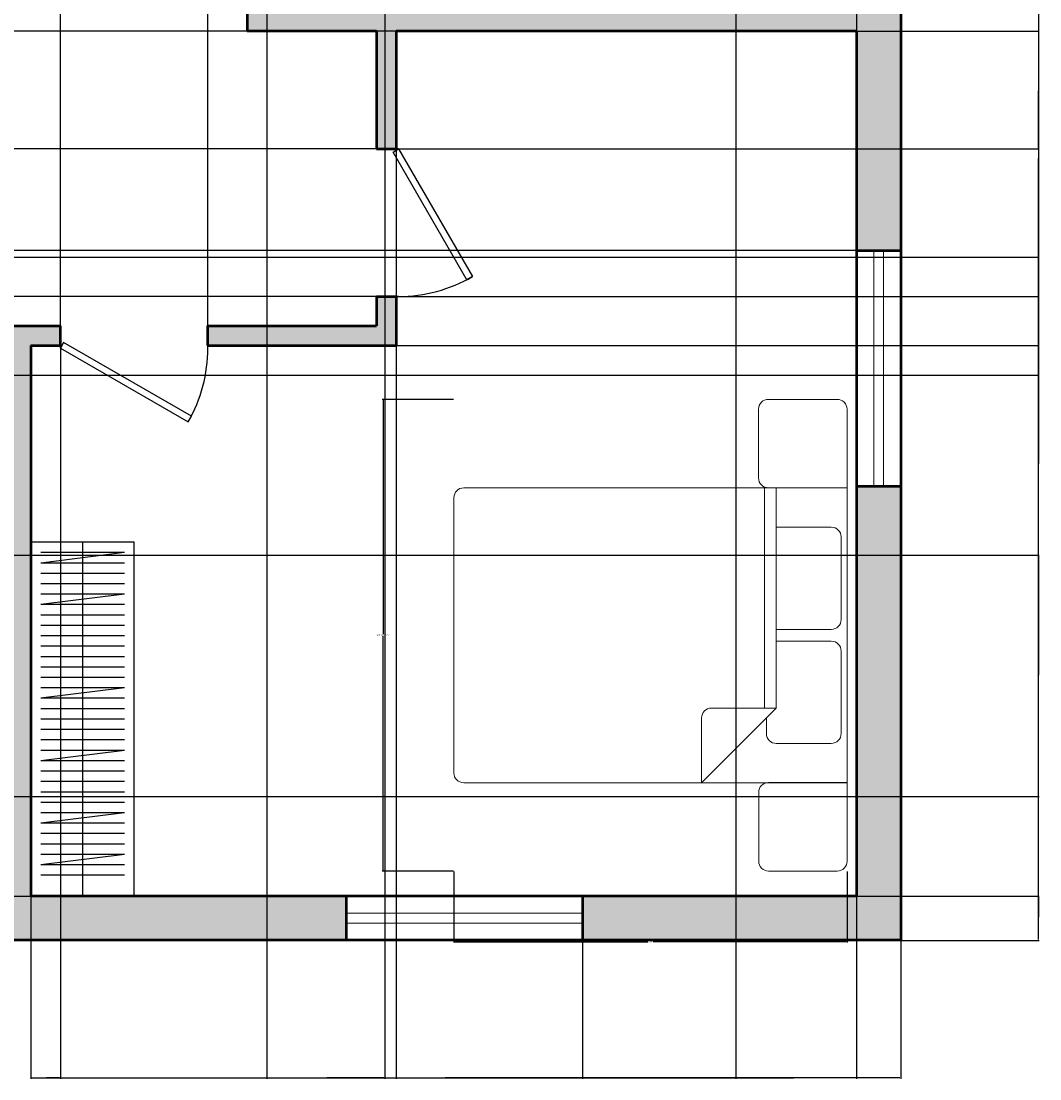
# Model space of a CAD drawing. Units: inches. Extents: x 1869 to 2483, y 2084 to 2479.
# Tile 6 of 7: x 2276 to 2483, y 2084 to 2299. Entities that reach past the tile are written whole.
import ezdxf

# ---------------------------------------------------------------- set-up
doc = ezdxf.new("R2010")
doc.units = ezdxf.units.IN
for name, color, linetype, lineweight in [('A-ANNO-DIMS', 2, 'Continuous', 18), ('A-DOOR', 3, 'Continuous', 25), ('A-FLOR-CASE', 9, 'Continuous', 25), ('A-FURN', 8, 'Continuous', 18), ('A-GLAZ', 4, 'Continuous', 18), ('A-WALL', 7, 'Continuous', 50)]:
    doc.layers.add(name, color=color, linetype=linetype, lineweight=lineweight)
doc.layers.add('A-WALL-PATT', color=18, linetype='Continuous', lineweight=13, true_color=0x000000)
doc.styles.get("Standard").update_dxf_attribs({"font": 'arial.ttf'})
doc.dimstyles.get("Standard").update_dxf_attribs({"dimtxt": 0.18, "dimasz": 0.18, "dimexe": 0.18, "dimexo": 0.0625, "dimgap": 0.09, "dimtad": 0, "dimtih": 1, "dimtoh": 1, "dimdec": 4, "dimzin": 0, "dimdsep": 46, "dimtxsty": 'Standard', "dimcen": 0.09, "dimadec": 0, "dimazin": 0, "dimtfac": 1, "dimtdec": 4, "dimtofl": 0, "dimtmove": 0, "dimatfit": 3, "dimfxl": 1, "dimtolj": 1, "dimtzin": 0, "dimarcsym": 0})

# ---------------------------------------------------------------- blocks, each defined once
blk = doc.blocks.new('Bed - Queen')
for p, q in [((0, -78), (0, 0)), ((0, 0), (60, 0)), ((60, 0), (60, -78)), ((10, -1.2), (26.8, -1.2)), ((33.2, -1.2), (50, -1.2)), ((8, -14.4), (8, -3.2)), ((28.8, -3.2), (28.8, -14.4)), ((31.2, -14.4), (31.2, -3.2)), ((52, -3.2), (52, -14.4)), ((0, -14.4), (44.8, -14.4)), ((60, -29.6), (44.8, -14.4)), ((44.8, -14.4), (44.8, -27.6)), ((44.8, -16.8), (0, -16.8)), ((50, -16.4), (46.8, -16.4)), ((46.8, -29.6), (60, -29.6)), ((58, -80), (2, -80))]:
    blk.add_line(p, q)
for points in [[(0, 0), (-16, 0, 0.414214), (-18, -2), (-18, -16, 0.414214), (-16, -18), (-2, -18, 0.414214), (0, -16)], [(75.96, 0.02), (59.96, 0.02), (59.96, -15.98, 0.414214), (61.96, -17.98), (75.96, -17.98, 0.414214), (77.96, -15.98), (77.96, -1.98, 0.414214)]]:
    blk.add_lwpolyline(points, format="xyb", close=True)
for centre, start, end in [((10, -3.2), 90, 180), ((26.8, -3.2), 0, 90), ((33.2, -3.2), 90, 180), ((50, -3.2), 0, 90), ((50, -14.4), 270, 0), ((46.8, -27.6), 180, 270), ((2, -78), 180, 270), ((58, -78), 270, 0)]:
    blk.add_arc(centre, 2, start, end)
blk = doc.blocks.new('*U13')
for p, q in [((0, 0), (0, 6)), ((40, 0), (40, 6))]:
    blk.add_line(p, q)
blk.add_lwpolyline([(0, 0), (34.64, -20), (35.52, -18.48), (0.87, 1.52)], close=True)
blk.add_arc((0, 0), 40, 330, 0)
blk = doc.blocks.new('*U10')
for p, q in [((0, 0), (0, -6)), ((40, 0), (40, -6))]:
    blk.add_line(p, q)
blk.add_lwpolyline([(0, 0), (34.64, 20), (35.52, 18.48), (0.87, -1.52)], close=True)
blk.add_arc((0, 0), 40, 0, 30)
blk = doc.blocks.new('WIN-GLAZING-48IN')
for p, q in [((0, 2), (48, 2)), ((0, 0), (48, 0))]:
    blk.add_line(p, q)
blk = doc.blocks.new('*D19')
at = {"layer": 'A-ANNO-DIMS', "color": 0, "lineweight": -2, "transparency": 16777216}
for p, q in [((2364.09, 2221.78), (2349.57, 2221.78)), ((2349.75, 2221.6), (2349.75, 2173.99)), ((2349.75, 2126), (2349.75, 2173.62)), ((2364.09, 2125.82), (2349.57, 2125.82))]:
    blk.add_line(p, q, dxfattribs=at)
at = {"layer": 'A-ANNO-DIMS', "color": 0, "transparency": 16777216}
for points in [[(2349.72, 2221.6), (2349.78, 2221.6), (2349.75, 2221.78)], [(2349.72, 2126), (2349.78, 2126), (2349.75, 2125.82)]]:
    blk.add_solid(points, dxfattribs=at)
at = {"layer": 'Defpoints', "color": 0, "transparency": 16777216}
for p in [(2364.15, 2221.78), (2349.75, 2125.82), (2364.15, 2125.82)]:
    blk.add_point(p, dxfattribs=at)
at = {"layer": 'A-ANNO-DIMS', "color": 0, "transparency": 16777216, "insert": (2349.75, 2173.8), "char_height": 0.18, "attachment_point": 5}
blk.add_mtext('\\A1;QUEEN BED SET 96 TYP.', dxfattribs=at)
blk = doc.blocks.new('*D20')
at = {"layer": 'A-ANNO-DIMS', "color": 0, "lineweight": -2, "transparency": 16777216}
for p, q in [((2364.15, 2125.76), (2364.15, 2111.25)), ((2444.17, 2125.76), (2444.17, 2111.25)), ((2364.33, 2111.43), (2403.63, 2111.43)), ((2443.99, 2111.43), (2404.69, 2111.43))]:
    blk.add_line(p, q, dxfattribs=at)
at = {"layer": 'A-ANNO-DIMS', "color": 0, "transparency": 16777216}
for points in [[(2364.33, 2111.46), (2364.33, 2111.4), (2364.15, 2111.43)], [(2443.99, 2111.46), (2443.99, 2111.4), (2444.17, 2111.43)]]:
    blk.add_solid(points, dxfattribs=at)
at = {"layer": 'Defpoints', "color": 0, "transparency": 16777216}
for p in [(2364.15, 2125.82), (2444.17, 2125.82), (2444.17, 2111.43)]:
    blk.add_point(p, dxfattribs=at)
at = {"layer": 'A-ANNO-DIMS', "color": 0, "transparency": 16777216, "insert": (2404.16, 2111.43), "char_height": 0.18, "attachment_point": 5}
blk.add_mtext('\\A1;80 TYP.', dxfattribs=at)
blk = doc.blocks.new('*D42')
at = {"layer": 'A-ANNO-DIMS', "color": 0, "lineweight": -2, "transparency": 16777216}
for p, q in [((2278.08, 2120.66), (2278.08, 2083.54)), ((2446.08, 2120.66), (2446.08, 2083.54)), ((2278.26, 2083.72), (2361.8, 2083.72)), ((2445.9, 2083.72), (2362.36, 2083.72))]:
    blk.add_line(p, q, dxfattribs=at)
at = {"layer": 'A-ANNO-DIMS', "color": 0, "transparency": 16777216}
for points in [[(2278.26, 2083.75), (2278.26, 2083.69), (2278.08, 2083.72)], [(2445.9, 2083.75), (2445.9, 2083.69), (2446.08, 2083.72)]]:
    blk.add_solid(points, dxfattribs=at)
at = {"layer": 'Defpoints', "color": 0, "transparency": 16777216}
for p in [(2278.08, 2120.72), (2446.08, 2120.72), (2446.08, 2083.72)]:
    blk.add_point(p, dxfattribs=at)
at = {"layer": 'A-ANNO-DIMS', "color": 0, "transparency": 16777216, "insert": (2362.08, 2083.72), "char_height": 0.18, "attachment_point": 5}
blk.add_mtext('\\A1;168', dxfattribs=at)
blk = doc.blocks.new('*D48')
at = {"layer": 'A-ANNO-DIMS', "color": 0, "lineweight": -2, "transparency": 16777216}
for p, q in [((2446.14, 2296.72), (2483.26, 2296.72)), ((2483.08, 2296.54), (2483.08, 2208.91)), ((2483.08, 2120.9), (2483.08, 2208.54)), ((2446.14, 2120.72), (2483.26, 2120.72))]:
    blk.add_line(p, q, dxfattribs=at)
at = {"layer": 'A-ANNO-DIMS', "color": 0, "transparency": 16777216}
for points in [[(2483.05, 2296.54), (2483.11, 2296.54), (2483.08, 2296.72)], [(2483.05, 2120.9), (2483.11, 2120.9), (2483.08, 2120.72)]]:
    blk.add_solid(points, dxfattribs=at)
at = {"layer": 'Defpoints', "color": 0, "transparency": 16777216}
for p in [(2446.08, 2296.72), (2483.08, 2296.72), (2446.08, 2120.72)]:
    blk.add_point(p, dxfattribs=at)
at = {"layer": 'A-ANNO-DIMS', "color": 0, "transparency": 16777216, "insert": (2483.08, 2208.72), "char_height": 0.18, "attachment_point": 5}
blk.add_mtext('\\A1;176', dxfattribs=at)
blk = doc.blocks.new('*D52')
at = {"layer": 'A-ANNO-DIMS', "color": 0, "lineweight": -2, "transparency": 16777216}
for p, q in [((2421.52, 2420.66), (2421.52, 2083.54)), ((2446.08, 2420.66), (2446.08, 2083.54)), ((2421.7, 2083.72), (2433.34, 2083.72)), ((2445.9, 2083.72), (2434.27, 2083.72))]:
    blk.add_line(p, q, dxfattribs=at)
at = {"layer": 'A-ANNO-DIMS', "color": 0, "transparency": 16777216}
for points in [[(2421.7, 2083.75), (2421.7, 2083.69), (2421.52, 2083.72)], [(2445.9, 2083.75), (2445.9, 2083.69), (2446.08, 2083.72)]]:
    blk.add_solid(points, dxfattribs=at)
at = {"layer": 'Defpoints', "color": 0, "transparency": 16777216}
for p in [(2421.52, 2420.72), (2446.08, 2420.72), (2446.08, 2083.72)]:
    blk.add_point(p, dxfattribs=at)
at = {"layer": 'A-ANNO-DIMS', "color": 0, "transparency": 16777216, "insert": (2433.8, 2083.72), "char_height": 0.18, "attachment_point": 5}
blk.add_mtext('\\A1;24.555', dxfattribs=at)
blk = doc.blocks.new('*D56')
at = {"layer": 'A-ANNO-DIMS', "color": 0, "lineweight": -2, "transparency": 16777216}
for p, q in [((2390.29, 2111.66), (2390.29, 2083.54)), ((2455.08, 2111.66), (2455.08, 2083.54)), ((2390.47, 2083.72), (2422.29, 2083.72)), ((2454.9, 2083.72), (2423.08, 2083.72))]:
    blk.add_line(p, q, dxfattribs=at)
at = {"layer": 'A-ANNO-DIMS', "color": 0, "transparency": 16777216}
for points in [[(2390.47, 2083.75), (2390.47, 2083.69), (2390.29, 2083.72)], [(2454.9, 2083.75), (2454.9, 2083.69), (2455.08, 2083.72)]]:
    blk.add_solid(points, dxfattribs=at)
at = {"layer": 'Defpoints', "color": 0, "transparency": 16777216}
for p in [(2390.29, 2111.72), (2455.08, 2111.72), (2455.08, 2083.72)]:
    blk.add_point(p, dxfattribs=at)
at = {"layer": 'A-ANNO-DIMS', "color": 0, "transparency": 16777216, "insert": (2422.68, 2083.72), "char_height": 0.18, "attachment_point": 5}
blk.add_mtext('\\A1;64.79', dxfattribs=at)
blk = doc.blocks.new('*D57')
at = {"layer": 'A-ANNO-DIMS', "color": 0, "lineweight": -2, "transparency": 16777216}
for p, q in [((2446.02, 2296.72), (1868.9, 2296.72)), ((1869.08, 2296.54), (1869.08, 2274.58)), ((1869.08, 2252.25), (1869.08, 2274.22)), ((2446.02, 2252.07), (1868.9, 2252.07))]:
    blk.add_line(p, q, dxfattribs=at)
at = {"layer": 'A-ANNO-DIMS', "color": 0, "transparency": 16777216}
for points in [[(1869.05, 2296.54), (1869.11, 2296.54), (1869.08, 2296.72)], [(1869.05, 2252.25), (1869.11, 2252.25), (1869.08, 2252.07)]]:
    blk.add_solid(points, dxfattribs=at)
at = {"layer": 'Defpoints', "color": 0, "transparency": 16777216}
for p in [(1869.08, 2296.72), (2446.08, 2296.72), (2446.08, 2252.07)]:
    blk.add_point(p, dxfattribs=at)
at = {"layer": 'A-ANNO-DIMS', "color": 0, "transparency": 16777216, "insert": (1869.08, 2274.4), "char_height": 0.18, "attachment_point": 5}
blk.add_mtext('\\A1;44.65', dxfattribs=at)
blk = doc.blocks.new('*D60')
at = {"layer": 'A-ANNO-DIMS', "color": 0, "lineweight": -2, "transparency": 16777216}
for p, q in [((2352.46, 2242.72), (2483.26, 2242.72)), ((2483.08, 2242.54), (2483.08, 2237.91)), ((2483.08, 2232.9), (2483.08, 2237.54)), ((2352.46, 2232.72), (2483.26, 2232.72))]:
    blk.add_line(p, q, dxfattribs=at)
at = {"layer": 'A-ANNO-DIMS', "color": 0, "transparency": 16777216}
for points in [[(2483.05, 2242.54), (2483.11, 2242.54), (2483.08, 2242.72)], [(2483.05, 2232.9), (2483.11, 2232.9), (2483.08, 2232.72)]]:
    blk.add_solid(points, dxfattribs=at)
at = {"layer": 'Defpoints', "color": 0, "transparency": 16777216}
for p in [(2352.4, 2242.72), (2483.08, 2242.72), (2352.4, 2232.72)]:
    blk.add_point(p, dxfattribs=at)
at = {"layer": 'A-ANNO-DIMS', "color": 0, "transparency": 16777216, "insert": (2483.08, 2237.72), "char_height": 0.18, "attachment_point": 5}
blk.add_mtext('\\A1;10', dxfattribs=at)
blk = doc.blocks.new('*D61')
at = {"layer": 'A-ANNO-DIMS', "color": 0, "lineweight": -2, "transparency": 16777216}
for p, q in [((2352.4, 2296.66), (2352.4, 2083.54)), ((2446.08, 2296.66), (2446.08, 2083.54)), ((2352.58, 2083.72), (2398.85, 2083.72)), ((2445.9, 2083.72), (2399.63, 2083.72))]:
    blk.add_line(p, q, dxfattribs=at)
at = {"layer": 'A-ANNO-DIMS', "color": 0, "transparency": 16777216}
for points in [[(2352.58, 2083.75), (2352.58, 2083.69), (2352.4, 2083.72)], [(2445.9, 2083.75), (2445.9, 2083.69), (2446.08, 2083.72)]]:
    blk.add_solid(points, dxfattribs=at)
at = {"layer": 'Defpoints', "color": 0, "transparency": 16777216}
for p in [(2352.4, 2296.72), (2446.08, 2296.72), (2446.08, 2083.72)]:
    blk.add_point(p, dxfattribs=at)
at = {"layer": 'A-ANNO-DIMS', "color": 0, "transparency": 16777216, "insert": (2399.24, 2083.72), "char_height": 0.18, "attachment_point": 5}
blk.add_mtext('\\A1;93.68', dxfattribs=at)
blk = doc.blocks.new('*D63')
at = {"layer": 'A-ANNO-DIMS', "color": 0, "lineweight": -2, "transparency": 16777216}
for p, q in [((2348.34, 2272.72), (1868.9, 2272.72)), ((1869.08, 2272.54), (1869.08, 2257.91)), ((1869.08, 2242.9), (1869.08, 2257.54)), ((2348.34, 2242.72), (1868.9, 2242.72))]:
    blk.add_line(p, q, dxfattribs=at)
at = {"layer": 'A-ANNO-DIMS', "color": 0, "transparency": 16777216}
for points in [[(1869.05, 2272.54), (1869.11, 2272.54), (1869.08, 2272.72)], [(1869.05, 2242.9), (1869.11, 2242.9), (1869.08, 2242.72)]]:
    blk.add_solid(points, dxfattribs=at)
at = {"layer": 'Defpoints', "color": 0, "transparency": 16777216}
for p in [(1869.08, 2272.72), (2348.4, 2272.72), (2348.4, 2242.72)]:
    blk.add_point(p, dxfattribs=at)
at = {"layer": 'A-ANNO-DIMS', "color": 0, "transparency": 16777216, "insert": (1869.08, 2257.72), "char_height": 0.18, "attachment_point": 5}
blk.add_mtext('\\A1;30', dxfattribs=at)
blk = doc.blocks.new('*D64')
at = {"layer": 'A-ANNO-DIMS', "color": 0, "lineweight": -2, "transparency": 16777216}
for p, q in [((2284.08, 2236.79), (2284.08, 2479.07)), ((2284.26, 2478.89), (2298.86, 2478.89)), ((2313.9, 2478.89), (2299.3, 2478.89)), ((2314.08, 2236.79), (2314.08, 2479.07))]:
    blk.add_line(p, q, dxfattribs=at)
at = {"layer": 'A-ANNO-DIMS', "color": 0, "transparency": 16777216}
for points in [[(2284.26, 2478.92), (2284.26, 2478.86), (2284.08, 2478.89)], [(2313.9, 2478.92), (2313.9, 2478.86), (2314.08, 2478.89)]]:
    blk.add_solid(points, dxfattribs=at)
at = {"layer": 'Defpoints', "color": 0, "transparency": 16777216}
for p in [(2314.08, 2478.89), (2284.08, 2236.72), (2314.08, 2236.72)]:
    blk.add_point(p, dxfattribs=at)
at = {"layer": 'A-ANNO-DIMS', "color": 0, "transparency": 16777216, "insert": (2299.08, 2478.89), "char_height": 0.18, "attachment_point": 5}
blk.add_mtext('\\A1;30', dxfattribs=at)
blk = doc.blocks.new('*D68')
at = {"layer": 'A-ANNO-DIMS', "color": 0, "lineweight": -2, "transparency": 16777216}
for p, q in [((2010.14, 2250.72), (2483.26, 2250.72)), ((2483.08, 2250.54), (2483.08, 2238.9)), ((2483.08, 2226.9), (2483.08, 2238.54)), ((2010.14, 2226.72), (2483.26, 2226.72))]:
    blk.add_line(p, q, dxfattribs=at)
at = {"layer": 'A-ANNO-DIMS', "color": 0, "transparency": 16777216}
for points in [[(2483.05, 2250.54), (2483.11, 2250.54), (2483.08, 2250.72)], [(2483.05, 2226.9), (2483.11, 2226.9), (2483.08, 2226.72)]]:
    blk.add_solid(points, dxfattribs=at)
at = {"layer": 'Defpoints', "color": 0, "transparency": 16777216}
for p in [(2010.08, 2250.72), (2483.08, 2250.72), (2010.08, 2226.72)]:
    blk.add_point(p, dxfattribs=at)
at = {"layer": 'A-ANNO-DIMS', "color": 0, "transparency": 16777216, "insert": (2483.08, 2238.72), "char_height": 0.18, "attachment_point": 5}
blk.add_mtext('\\A1;24', dxfattribs=at)
blk = doc.blocks.new('*D73')
at = {"layer": 'A-ANNO-DIMS', "color": 0, "lineweight": -2, "transparency": 16777216}
for p, q in [((2200.14, 2120.72), (2483.26, 2120.72)), ((2483.08, 2120.54), (2483.08, 2116.41)), ((2483.08, 2111.9), (2483.08, 2116.04)), ((2200.14, 2111.72), (2483.26, 2111.72))]:
    blk.add_line(p, q, dxfattribs=at)
at = {"layer": 'A-ANNO-DIMS', "color": 0, "transparency": 16777216}
for points in [[(2483.05, 2120.54), (2483.11, 2120.54), (2483.08, 2120.72)], [(2483.05, 2111.9), (2483.11, 2111.9), (2483.08, 2111.72)]]:
    blk.add_solid(points, dxfattribs=at)
at = {"layer": 'Defpoints', "color": 0, "transparency": 16777216}
for p in [(2200.08, 2120.72), (2483.08, 2120.72), (2200.08, 2111.72)]:
    blk.add_point(p, dxfattribs=at)
at = {"layer": 'A-ANNO-DIMS', "color": 0, "transparency": 16777216, "insert": (2483.08, 2116.22), "char_height": 0.18, "attachment_point": 5}
blk.add_mtext('\\A1;9', dxfattribs=at)
blk = doc.blocks.new('*D76')
at = {"layer": 'A-ANNO-DIMS', "color": 0, "lineweight": -2, "transparency": 16777216}
for p, q in [((2455.14, 2429.72), (2483.26, 2429.72)), ((2483.08, 2429.54), (2483.08, 2270.91)), ((2483.08, 2111.9), (2483.08, 2270.54)), ((2455.14, 2111.72), (2483.26, 2111.72))]:
    blk.add_line(p, q, dxfattribs=at)
at = {"layer": 'A-ANNO-DIMS', "color": 0, "transparency": 16777216}
for points in [[(2483.05, 2429.54), (2483.11, 2429.54), (2483.08, 2429.72)], [(2483.05, 2111.9), (2483.11, 2111.9), (2483.08, 2111.72)]]:
    blk.add_solid(points, dxfattribs=at)
at = {"layer": 'Defpoints', "color": 0, "transparency": 16777216}
for p in [(2455.08, 2429.72), (2483.08, 2429.72), (2455.08, 2111.72)]:
    blk.add_point(p, dxfattribs=at)
at = {"layer": 'A-ANNO-DIMS', "color": 0, "transparency": 16777216, "insert": (2483.08, 2270.72), "char_height": 0.18, "attachment_point": 5}
blk.add_mtext('\\A1;318', dxfattribs=at)
blk = doc.blocks.new('*D77')
at = {"layer": 'A-ANNO-DIMS', "color": 0, "lineweight": -2, "transparency": 16777216}
for p, q in [((2326.08, 2336.66), (2326.08, 2083.54)), ((2350.08, 2336.66), (2350.08, 2083.54)), ((2326.26, 2083.72), (2337.86, 2083.72)), ((2349.9, 2083.72), (2338.3, 2083.72))]:
    blk.add_line(p, q, dxfattribs=at)
at = {"layer": 'A-ANNO-DIMS', "color": 0, "transparency": 16777216}
for points in [[(2326.26, 2083.75), (2326.26, 2083.69), (2326.08, 2083.72)], [(2349.9, 2083.75), (2349.9, 2083.69), (2350.08, 2083.72)]]:
    blk.add_solid(points, dxfattribs=at)
at = {"layer": 'Defpoints', "color": 0, "transparency": 16777216}
for p in [(2326.08, 2336.72), (2350.08, 2336.72), (2350.08, 2083.72)]:
    blk.add_point(p, dxfattribs=at)
at = {"layer": 'A-ANNO-DIMS', "color": 0, "transparency": 16777216, "insert": (2338.08, 2083.72), "char_height": 0.18, "attachment_point": 5}
blk.add_mtext('\\A1;24', dxfattribs=at)
blk = doc.blocks.new('*D80')
at = {"layer": 'A-ANNO-DIMS', "color": 0, "lineweight": -2, "transparency": 16777216}
for p, q in [((2278.08, 2232.66), (2278.08, 2083.54)), ((2284.08, 2232.66), (2284.08, 2083.54)), ((2278.26, 2083.72), (2280.93, 2083.72)), ((2283.9, 2083.72), (2281.23, 2083.72))]:
    blk.add_line(p, q, dxfattribs=at)
at = {"layer": 'A-ANNO-DIMS', "color": 0, "transparency": 16777216}
for points in [[(2278.26, 2083.75), (2278.26, 2083.69), (2278.08, 2083.72)], [(2283.9, 2083.75), (2283.9, 2083.69), (2284.08, 2083.72)]]:
    blk.add_solid(points, dxfattribs=at)
at = {"layer": 'Defpoints', "color": 0, "transparency": 16777216}
for p in [(2278.08, 2232.72), (2284.08, 2232.72), (2284.08, 2083.72)]:
    blk.add_point(p, dxfattribs=at)
at = {"layer": 'A-ANNO-DIMS', "color": 0, "transparency": 16777216, "insert": (2281.08, 2083.72), "char_height": 0.18, "attachment_point": 5}
blk.add_mtext('\\A1;6', dxfattribs=at)
blk = doc.blocks.new('*D81')
at = {"layer": 'A-ANNO-DIMS', "color": 0, "lineweight": -2, "transparency": 16777216}
for p, q in [((2352.46, 2296.72), (2483.26, 2296.72)), ((2483.08, 2296.54), (2483.08, 2284.9)), ((2483.08, 2272.9), (2483.08, 2284.54)), ((2352.46, 2272.72), (2483.26, 2272.72))]:
    blk.add_line(p, q, dxfattribs=at)
at = {"layer": 'A-ANNO-DIMS', "color": 0, "transparency": 16777216}
for points in [[(2483.05, 2296.54), (2483.11, 2296.54), (2483.08, 2296.72)], [(2483.05, 2272.9), (2483.11, 2272.9), (2483.08, 2272.72)]]:
    blk.add_solid(points, dxfattribs=at)
at = {"layer": 'Defpoints', "color": 0, "transparency": 16777216}
for p in [(2352.4, 2296.72), (2483.08, 2296.72), (2352.4, 2272.72)]:
    blk.add_point(p, dxfattribs=at)
at = {"layer": 'A-ANNO-DIMS', "color": 0, "transparency": 16777216, "insert": (2483.08, 2284.72), "char_height": 0.18, "attachment_point": 5}
blk.add_mtext('\\A1;24', dxfattribs=at)
blk = doc.blocks.new('*D93')
at = {"layer": 'A-ANNO-DIMS', "color": 0, "lineweight": -2, "transparency": 16777216}
for p, q in [((2103.9, 2190.06), (2483.26, 2190.06)), ((2483.08, 2189.88), (2483.08, 2165.72)), ((2483.08, 2141.19), (2483.08, 2165.36)), ((2103.9, 2141.01), (2483.26, 2141.01))]:
    blk.add_line(p, q, dxfattribs=at)
at = {"layer": 'A-ANNO-DIMS', "color": 0, "transparency": 16777216}
for points in [[(2483.05, 2189.88), (2483.11, 2189.88), (2483.08, 2190.06)], [(2483.05, 2141.19), (2483.11, 2141.19), (2483.08, 2141.01)]]:
    blk.add_solid(points, dxfattribs=at)
at = {"layer": 'Defpoints', "color": 0, "transparency": 16777216}
for p in [(2103.84, 2190.06), (2483.08, 2190.06), (2103.84, 2141.01)]:
    blk.add_point(p, dxfattribs=at)
at = {"layer": 'A-ANNO-DIMS', "color": 0, "transparency": 16777216, "insert": (2483.08, 2165.54), "char_height": 0.18, "attachment_point": 5}
blk.add_mtext('\\A1;49.05', dxfattribs=at)

msp = doc.modelspace()

# ---------------------------------------------------------------- hatches: boundary and pattern name
at = {"layer": 'A-WALL-PATT'}
h = msp.add_hatch(color=256, dxfattribs=at)
h.dxf.hatch_style = 1
h.paths.add_polyline_path([(2352.3982, 2296.7235), (2446.0799, 2296.7235), (2446.0799, 2252.0706), (2455.0799, 2252.0706), (2455.0799, 2429.7235), (2421.5248, 2429.7235), (2421.5248, 2420.7235), (2446.0799, 2420.7235), (2446.0799, 2300.7235), (2326.0799, 2300.7235), (2326.0799, 2306.7235), (2322.0799, 2306.7235), (2322.0799, 2296.7235), (2348.3982, 2296.7235), (2348.3982, 2272.7235), (2352.3982, 2272.7235)])
h = msp.add_hatch(color=256, dxfattribs=at)
h.dxf.hatch_style = 1
h.paths.add_polyline_path([(2352.3982, 2242.7235), (2348.3982, 2242.7235), (2348.3982, 2236.7235), (2314.0799, 2236.7235), (2314.0799, 2232.7235), (2352.3982, 2232.7235)])
h = msp.add_hatch(color=256, dxfattribs=at)
h.dxf.hatch_style = 1
h.paths.add_polyline_path([(2342.287, 2120.7235), (2278.0799, 2120.7235), (2278.0799, 2192.7235), (2278.0799, 2232.7235), (2284.0799, 2232.7235), (2284.0799, 2236.7235), (2274.0799, 2236.7235), (2274.0799, 2120.7235), (2200.0799, 2120.7235), (2200.0799, 2111.7235), (2342.287, 2111.7235)])
h = msp.add_hatch(color=256, dxfattribs=at)
h.dxf.hatch_style = 1
h.paths.add_polyline_path([(2455.0799, 2204.0706), (2446.0799, 2204.0706), (2446.0799, 2120.7235), (2390.287, 2120.7235), (2390.287, 2111.7235), (2455.0799, 2111.7235)])

# ---------------------------------------------------------------- linework, layer by layer
at = {"layer": 'A-FLOR-CASE'}
for p, q in [((2299.0799, 2192.7235), (2278.0799, 2192.7235)), ((2288.5799, 2192.7235), (2288.5799, 2120.7235)), ((2299.0799, 2120.7235), (2299.0799, 2192.7235)), ((2297.0799, 2190.6059), (2280.0799, 2190.6059)), ((2297.0799, 2190.6059), (2280.0799, 2188.4882)), ((2297.0799, 2188.4882), (2280.0799, 2188.4882)), ((2297.0799, 2186.3706), (2280.0799, 2186.3706)), ((2297.0799, 2184.2529), (2280.0799, 2184.2529)), ((2297.0799, 2182.1353), (2280.0799, 2182.1353)), ((2297.0799, 2182.1353), (2280.0799, 2180.0176)), ((2297.0799, 2180.0176), (2280.0799, 2180.0176)), ((2297.0799, 2177.9), (2280.0799, 2177.9)), ((2297.0799, 2175.7824), (2280.0799, 2175.7824)), ((2297.0799, 2173.6647), (2280.0799, 2173.6647)), ((2297.0799, 2171.5471), (2280.0799, 2171.5471)), ((2297.0799, 2169.4294), (2280.0799, 2169.4294)), ((2297.0799, 2167.3118), (2280.0799, 2167.3118)), ((2297.0799, 2165.1941), (2280.0799, 2165.1941)), ((2297.0799, 2163.0765), (2280.0799, 2163.0765)), ((2297.0799, 2163.0765), (2280.0799, 2160.9588)), ((2297.0799, 2160.9588), (2280.0799, 2160.9588)), ((2297.0799, 2158.8412), (2280.0799, 2158.8412)), ((2297.0799, 2156.7235), (2280.0799, 2156.7235)), ((2297.0799, 2154.6059), (2280.0799, 2154.6059)), ((2297.0799, 2152.4882), (2280.0799, 2152.4882)), ((2297.0799, 2150.3706), (2280.0799, 2150.3706)), ((2297.0799, 2150.3706), (2280.0799, 2148.2529)), ((2297.0799, 2148.2529), (2280.0799, 2148.2529)), ((2297.0799, 2146.1353), (2280.0799, 2146.1353)), ((2297.0799, 2144.0176), (2280.0799, 2144.0176)), ((2297.0799, 2141.9), (2280.0799, 2141.9)), ((2297.0799, 2139.7824), (2280.0799, 2139.7824)), ((2297.0799, 2137.6647), (2280.0799, 2137.6647)), ((2297.0799, 2137.6647), (2280.0799, 2135.5471)), ((2297.0799, 2135.5471), (2280.0799, 2135.5471)), ((2297.0799, 2133.4294), (2280.0799, 2133.4294)), ((2297.0799, 2131.3118), (2280.0799, 2131.3118)), ((2297.0799, 2129.1941), (2280.0799, 2129.1941)), ((2297.0799, 2129.1941), (2280.0799, 2127.0765)), ((2297.0799, 2127.0765), (2280.0799, 2127.0765)), ((2297.0799, 2124.9588), (2280.0799, 2124.9588)), ((2278.0799, 2120.7235), (2299.0799, 2120.7235)), ((2299.0799, 2120.7235), (2278.0799, 2120.7235))]:
    msp.add_line(p, q, dxfattribs=at)
at = {"layer": 'A-WALL'}
for p, q in [((2322.0799, 2306.7235), (2322.0799, 2296.7235)), ((2322.0799, 2296.7235), (2348.3982, 2296.7235)), ((2348.3982, 2296.7235), (2348.3982, 2272.7235)), ((2352.3982, 2296.7235), (2352.3982, 2272.7235)), ((2352.3982, 2296.7235), (2446.0799, 2296.7235)), ((2446.0799, 2296.7235), (2446.0799, 2120.7235)), ((2348.3982, 2272.7235), (2352.3982, 2272.7235)), ((2446.0799, 2252.0706), (2455.0799, 2252.0706)), ((2348.3982, 2242.7235), (2352.3982, 2242.7235)), ((2348.3982, 2242.7235), (2348.3982, 2236.7235)), ((2352.3982, 2242.7235), (2352.3982, 2232.7235)), ((2274.0799, 2236.7235), (2284.0799, 2236.7235)), ((2284.0799, 2232.7235), (2284.0799, 2236.7235)), ((2314.0799, 2232.7235), (2314.0799, 2236.7235)), ((2314.0799, 2236.7235), (2348.3982, 2236.7235)), ((2278.0799, 2232.7235), (2278.0799, 2120.7235)), ((2278.0799, 2232.7235), (2284.0799, 2232.7235)), ((2314.0799, 2232.7235), (2352.3982, 2232.7235)), ((2455.0799, 2204.0706), (2446.0799, 2204.0706)), ((2278.0799, 2192.7235), (2278.0799, 2120.7235)), ((2446.0799, 2120.7235), (2278.0799, 2120.7235)), ((2342.287, 2111.7235), (2342.287, 2120.7235)), ((2390.287, 2120.7235), (2390.287, 2111.7235))]:
    msp.add_line(p, q, dxfattribs=at)
msp.add_lwpolyline([(2152.0799, 2111.7235), (1897.0799, 2111.7235), (1897.0799, 2429.7235), (2455.0799, 2429.7235), (2455.0799, 2111.7235), (2200.0799, 2111.7235)], dxfattribs=at)

# ---------------------------------------------------------------- block references
at = {"layer": 'A-DOOR', "xscale": 0.75, "yscale": 0.75, "zscale": 0.75, "rotation": 270}
msp.add_blockref('*U10', (2352.8982, 2272.7235), dxfattribs=at)
at = {"layer": 'A-DOOR', "xscale": 0.75, "yscale": 0.75, "zscale": 0.75}
msp.add_blockref('*U13', (2284.0799, 2232.2235), dxfattribs=at)
at = {"layer": 'A-FURN', "rotation": 270}
msp.add_blockref('Bed - Queen', (2444.1479, 2203.7836), dxfattribs=at)
at = {"layer": 'A-GLAZ', "rotation": 90.00000000000003}
msp.add_blockref('WIN-GLAZING-48IN', (2451.5794, 2204.0705), dxfattribs=at)
at = {"layer": 'A-GLAZ'}
msp.add_blockref('WIN-GLAZING-48IN', (2342.2869, 2115.224), dxfattribs=at)

# ---------------------------------------------------------------- dimensions: what is measured, and where the dimension line sits
at = {"layer": 'A-ANNO-DIMS'}
for base, p1, p2, override, picture, middle in [((2314.0799, 2478.8871), (2284.0799, 2236.7235), (2314.0799, 2236.7235), {"dimdec": 0, "dimlfac": 1, "dimrnd": 0, "dimzin": 0, "dimdsep": 46, "dimlunit": 2}, '*D64', (2299.0799, 2478.8871)), ((2446.0799, 2083.7235), (2421.5248, 2420.7235), (2446.0799, 2420.7235), {"dimdec": 3, "dimlfac": 1, "dimrnd": 0, "dimzin": 0, "dimdsep": 46, "dimlunit": 2}, '*D52', (2433.8023, 2083.7235)), ((2350.0799, 2083.7235), (2326.0799, 2336.7235), (2350.0799, 2336.7235), {"dimdec": 0, "dimlfac": 1, "dimrnd": 0, "dimzin": 0, "dimdsep": 46, "dimlunit": 2}, '*D77', (2338.0799, 2083.7235)), ((2446.0799, 2083.7235), (2352.3982, 2296.7235), (2446.0799, 2296.7235), {"dimdec": 2, "dimlfac": 1, "dimrnd": 0, "dimzin": 0, "dimdsep": 46, "dimlunit": 2}, '*D61', (2399.239, 2083.7235)), ((2284.0799, 2083.7235), (2278.0799, 2232.7235), (2284.0799, 2232.7235), {"dimdec": 0, "dimlfac": 1, "dimrnd": 0, "dimzin": 0, "dimdsep": 46, "dimlunit": 2}, '*D80', (2281.0799, 2083.7235)), ((2446.0799, 2083.7235), (2278.0799, 2120.7235), (2446.0799, 2120.7235), {"dimdec": 0, "dimlfac": 1, "dimrnd": 0, "dimzin": 0, "dimdsep": 46, "dimlunit": 2}, '*D42', (2362.0799, 2083.7235)), ((2455.0799, 2083.7235), (2390.287, 2111.7235), (2455.0799, 2111.7235), {"dimdec": 2, "dimlfac": 1, "dimrnd": 0, "dimzin": 0, "dimdsep": 46, "dimlunit": 2}, '*D56', (2422.6835, 2083.7235))]:
    dim = msp.add_linear_dim(base=base, p1=p1, p2=p2, dimstyle='Standard', override=override, dxfattribs=at)
    dim.commit()
    dim.dimension.update_dxf_attribs({"geometry": picture, "text_midpoint": middle})
for base, p1, p2, override, picture, middle in [((2483.0799, 2429.7235), (2455.0799, 2111.7235), (2455.0799, 2429.7235), {"dimdec": 0, "dimlfac": 1, "dimrnd": 0, "dimzin": 0, "dimdsep": 46, "dimlunit": 2}, '*D76', (2483.0799, 2270.7235)), ((1869.0799, 2296.7235), (2446.0799, 2252.0706), (2446.0799, 2296.7235), {"dimdec": 2, "dimlfac": 1, "dimrnd": 0, "dimzin": 0, "dimdsep": 46, "dimlunit": 2}, '*D57', (1869.0799, 2274.3971)), ((2483.0799, 2296.7235), (2352.3982, 2272.7235), (2352.3982, 2296.7235), {"dimdec": 0, "dimlfac": 1, "dimrnd": 0, "dimzin": 0, "dimdsep": 46, "dimlunit": 2}, '*D81', (2483.0799, 2284.7235)), ((2483.0799, 2296.7235), (2446.0799, 2120.7235), (2446.0799, 2296.7235), {"dimdec": 0, "dimlfac": 1, "dimrnd": 0, "dimzin": 0, "dimdsep": 46, "dimlunit": 2}, '*D48', (2483.0799, 2208.7235)), ((1869.0799, 2272.7235), (2348.3982, 2242.7235), (2348.3982, 2272.7235), {"dimdec": 0, "dimlfac": 1, "dimrnd": 0, "dimzin": 0, "dimdsep": 46, "dimlunit": 2}, '*D63', (1869.0799, 2257.7235)), ((2483.0799, 2250.7235), (2010.0799, 2226.7235), (2010.0799, 2250.7235), {"dimdec": 0, "dimlfac": 1, "dimrnd": 0, "dimzin": 0, "dimdsep": 46, "dimlunit": 2}, '*D68', (2483.0799, 2238.7235)), ((2483.0799, 2242.7235), (2352.3982, 2232.7235), (2352.3982, 2242.7235), {"dimdec": 0, "dimlfac": 1, "dimrnd": 0, "dimzin": 0, "dimdsep": 46, "dimlunit": 2}, '*D60', (2483.0799, 2237.7235)), ((2483.0799, 2190.0613), (2103.8391, 2141.0143), (2103.8391, 2190.0613), {"dimdec": 2, "dimlfac": 1, "dimrnd": 0, "dimzin": 0, "dimdsep": 46, "dimlunit": 2}, '*D93', (2483.0799, 2165.5378)), ((2483.0799, 2120.7235), (2200.0799, 2111.7235), (2200.0799, 2120.7235), {"dimdec": 0, "dimlfac": 1, "dimrnd": 0, "dimzin": 0, "dimdsep": 46, "dimlunit": 2}, '*D73', (2483.0799, 2116.2235))]:
    dim = msp.add_linear_dim(base=base, p1=p1, p2=p2, angle=90, dimstyle='Standard', override=override, dxfattribs=at)
    dim.commit()
    dim.dimension.update_dxf_attribs({"geometry": picture, "text_midpoint": middle})
dim = msp.add_linear_dim(base=(2349.754, 2125.8244), p1=(2364.1479, 2221.7836), p2=(2364.1479, 2125.8244), angle=270, text='QUEEN BED SET <> TYP.', dimstyle='Standard', override={"dimdec": 0, "dimlfac": 1, "dimrnd": 0, "dimzin": 0, "dimdsep": 46, "dimlunit": 2}, dxfattribs=at)
dim.commit()
dim.dimension.update_dxf_attribs({"geometry": '*D19', "text_midpoint": (2349.754, 2173.804)})
dim = msp.add_linear_dim(base=(2444.17, 2111.4306), p1=(2364.1479, 2125.8244), p2=(2444.17, 2125.8244), text='<> TYP.', dimstyle='Standard', override={"dimdec": 0, "dimlfac": 1, "dimrnd": 0, "dimzin": 0, "dimdsep": 46, "dimlunit": 2}, dxfattribs=at)
dim.commit()
dim.dimension.update_dxf_attribs({"geometry": '*D20', "text_midpoint": (2404.1589, 2111.4306)})

doc.saveas('drawing.dxf')
